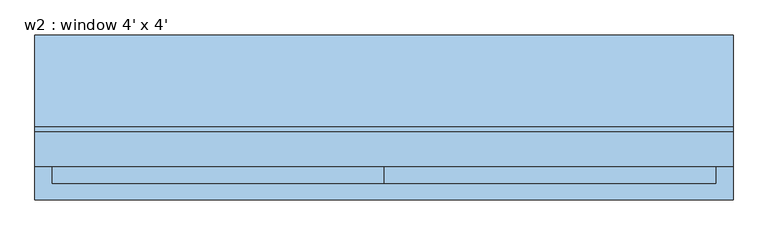
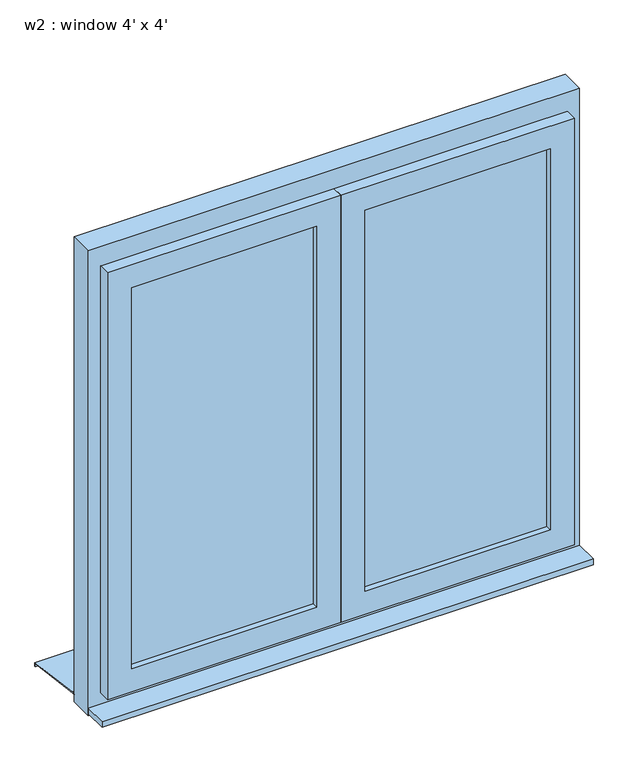
"""IFC4 building model written with IfcOpenShell, lengths in millimetres: window geometry, w2 : window 4' x 4'."""

from ifc_helpers import new_model, si_unit, frame, origin, place, context, project, spatial, polyline, outline, extrude, faceted_brep, source, transform, mapped, element, save


def w2_window_4_x_4_9dec5fc7(model_context):
    return source(origin(), model_context, "Body", "SolidModel", [
        extrude(outline(polyline([(-15.6778457, 1020.0), (144.3, 1000.0), (144.3, 990.0), (142.3, 990.0), (142.3, 998.3604634), (-15.8759277, 1018.0), (-25.7, 1018.0), (-25.7, 1020.0), (-15.6778457, 1020.0)])), frame((-609.6, 0.0, 0.0), z_axis=(1.0, 0.0, 0.0), x_axis=(0.0, 1.0, 0.0)), (0.0, 0.0, 1.0), 1219.2),
        extrude(outline(polyline([(-609.6, -144.3), (-609.6, -85.7), (609.6, -85.7), (609.6, -144.3), (-609.6, -144.3)])), frame((0.0, 0.0, 1005.0), z_axis=(0.0, 0.0, 1.0), x_axis=(1.0, 0.0, 0.0)), (0.0, 0.0, 1.0), 15.0),
        extrude(outline(polyline([(60.0, -70.7), (519.6, -70.7), (519.6, -100.7), (60.0, -100.7), (60.0, -70.7)])), frame((0.0, 0.0, 1110.0), z_axis=(0.0, 0.0, 1.0), x_axis=(1.0, 0.0, 0.0)), (0.0, 0.0, 1.0), 999.2),
        extrude(outline(polyline([(-519.6, -70.7), (-60.0, -70.7), (-60.0, -100.7), (-519.6, -100.7), (-519.6, -70.7)])), frame((0.0, 0.0, 1110.0), z_axis=(0.0, 0.0, 1.0), x_axis=(1.0, 0.0, 0.0)), (0.0, 0.0, 1.0), 999.2),
        extrude(outline(polyline([(2219.2, -609.6), (1000.0, -609.6), (1000.0, 609.6), (2219.2, 609.6), (2219.2, -609.6)]), holes=[polyline([(2139.2, -549.6), (2139.2, 549.6), (1080.0, 549.6), (1080.0, -549.6), (2139.2, -549.6)])]), frame((0.0, -85.7, 0.0), z_axis=(0.0, 1.0, 0.0), x_axis=(0.0, 0.0, 1.0)), (0.0, 0.0, 1.0), 60.0),
        extrude(outline(polyline([(30.0, -85.7), (-30.0, -85.7), (-30.0, -25.7), (30.0, -25.7), (30.0, -85.7)])), frame((0.0, 0.0, 1080.0), z_axis=(0.0, 0.0, 1.0), x_axis=(1.0, 0.0, 0.0)), (0.0, 0.0, 1.0), 1059.2),
        faceted_brep([(30.0, -85.7, 1080.0), (30.0, -55.7, 1080.0), (549.6, -55.7, 1080.0), (549.6, -85.7, 1080.0), (549.6, -55.7, 2139.2), (549.6, -85.7, 2139.2), (30.0, -55.7, 2139.2), (519.6, -55.7, 2109.2), (60.0, -55.7, 2109.2), (60.0, -55.7, 1110.0), (519.6, -55.7, 1110.0), (579.6, -85.7, 1050.0), (0.0, -85.7, 1050.0), (0.0, -85.7, 2169.2), (579.6, -85.7, 2169.2), (30.0, -85.7, 2139.2), (0.0, -115.7, 1050.0), (579.6, -115.7, 1050.0), (579.6, -115.7, 2169.2), (0.0, -115.7, 2169.2), (519.6, -115.7, 1110.0), (60.0, -115.7, 1110.0), (60.0, -115.7, 2109.2), (519.6, -115.7, 2109.2)], [[[0, 1, 2, 3]], [[3, 2, 4, 5]], [[2, 1, 6, 4], [7, 8, 9, 10]], [[11, 12, 13, 14], [5, 15, 0, 3]], [[16, 12, 11, 17]], [[17, 11, 14, 18]], [[18, 19, 16, 17], [20, 21, 22, 23]], [[9, 21, 20, 10]], [[10, 20, 23, 7]], [[15, 6, 1, 0]], [[19, 13, 12, 16]], [[8, 22, 21, 9]], [[5, 4, 6, 15]], [[18, 14, 13, 19]], [[7, 23, 22, 8]]]),
        faceted_brep([(-549.6, -85.7, 1080.0), (-549.6, -55.7, 1080.0), (-30.0, -55.7, 1080.0), (-30.0, -85.7, 1080.0), (-30.0, -55.7, 2139.2), (-30.0, -85.7, 2139.2), (-549.6, -55.7, 2139.2), (-60.0, -55.7, 2109.2), (-519.6, -55.7, 2109.2), (-519.6, -55.7, 1110.0), (-60.0, -55.7, 1110.0), (0.0, -85.7, 1050.0), (-579.6, -85.7, 1050.0), (-579.6, -85.7, 2169.2), (0.0, -85.7, 2169.2), (-549.6, -85.7, 2139.2), (-579.6, -115.7, 1050.0), (0.0, -115.7, 1050.0), (0.0, -115.7, 2169.2), (-579.6, -115.7, 2169.2), (-60.0, -115.7, 1110.0), (-519.6, -115.7, 1110.0), (-519.6, -115.7, 2109.2), (-60.0, -115.7, 2109.2)], [[[0, 1, 2, 3]], [[3, 2, 4, 5]], [[2, 1, 6, 4], [7, 8, 9, 10]], [[11, 12, 13, 14], [5, 15, 0, 3]], [[16, 12, 11, 17]], [[17, 11, 14, 18]], [[18, 19, 16, 17], [20, 21, 22, 23]], [[9, 21, 20, 10]], [[10, 20, 23, 7]], [[15, 6, 1, 0]], [[19, 13, 12, 16]], [[8, 22, 21, 9]], [[5, 4, 6, 15]], [[18, 14, 13, 19]], [[7, 23, 22, 8]]]),
    ])


if __name__ == "__main__":
    model = new_model("IFC4")
    model_context = context("Model", 3, world=origin())
    ifc_project = project(units=[si_unit("LENGTHUNIT", "METRE", prefix="MILLI")], contexts=[model_context])
    site = spatial("IfcSite", under=ifc_project)
    building = spatial("IfcBuilding", under=site)
    placement = place(None, origin())
    w2_window_4_x_4_shape = w2_window_4_x_4_9dec5fc7(model_context)
    element("IfcWindow", 1, ObjectType="w2 : window 4' x 4'", at=placement, inside=building, context=model_context, shape_type="MappedRepresentation", body=[
        mapped(w2_window_4_x_4_shape, transform((0.0, 0.0, 0.0), x_axis=(1.0, 0.0, 0.0), y_axis=(0.0, 1.0, 0.0), z_axis=(0.0, 0.0, 1.0))),
    ])
    save(model, "model.ifc")

# Revit data of these elements
# Type "w2 : window 4' x 4'"
#   Type Mark = "25"
#   Operation = "DoublePanelVertical"
#   Keynote = "16.05.01"
#   Analytic Construction = "<None>"
#   Rough Width = 4' - 0"
#   Rough Height = 4' - 0"
#   Rahmentiefe = 0' - 2.3622"
#   Rahmenhöhe unten = 0' - 3.14961"
#   Rahmehöhe oben = 0' - 3.14961"
#   Rahmenbreite = 0' - 2.3622"
#   Heat Transfer Coefficient (U) = 2.81836 BTU/(h·ft²·°F)
#   Height = 4' - 0"
#   Flügeltiefe = 0' - 2.3622"
#   Flügelbreite = 0' - 2.3622"
#   Einbautiefe (von außen) [instance default] = 0' - 5.51181"
#   Width = 4' - 0"
#   Kippflügel [instance default] = yes
#   Drehflügel im Grundriß darstellen [instance default] = no
#   Drehflügel [instance default] = yes
#   Define Thermal Properties by = 1
#   Rahmen [instance default] = none
#   Glas [instance default] = blue glass
#   Flügel [instance default] = WINDOW COLOUR WHITE
#   Fensterbank aussen [instance default] = WINDOW COLOUR WHITE
#   Fensterbank innen [instance default] = WINDOW COLOUR WHITE
#   Visual Light Transmittance = 0
#   Thermal Resistance (R) = 0
#   Solar Heat Gain Coefficient = 0
#   Wall Closure = (empty or 0)
# Element 1 (IfcWindow, "w2 : window 4' x 4'")
#   Materials on its faces: "WINDOW COLOUR WHITE", "blue glass"
# Materials
#   "blue glass": class "System", colour RGB 0 0 255, transparency 0.75, Cost = 0
#   "WINDOW COLOUR WHITE": class "Generic", colour RGB 120 120 120, transparency 0, Cost = 0
